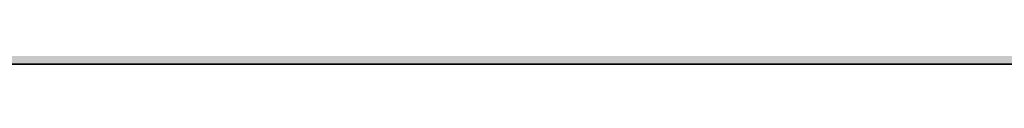
# Model space of a CAD drawing. Units: inches. Extents: x 2091 to 2899, y 967 to 2217.
# Tile 41 of 256: x 2390 to 2461, y 1091 to 1091. Entities that reach past the tile are written whole.
import ezdxf

# ---------------------------------------------------------------- set-up
doc = ezdxf.new("R2010")
doc.units = ezdxf.units.IN
doc.layers.add('A-WALL-PATT', color=141, linetype='Continuous', lineweight=13, true_color=0xadddf7)
doc.layers.add('C-PROP', color=7, linetype='Continuous', lineweight=35)

msp = doc.modelspace()

# ---------------------------------------------------------------- hatches: boundary and pattern name
at = {"layer": 'A-WALL-PATT'}
h = msp.add_hatch(color=256, dxfattribs=at)
h.dxf.hatch_style = 1
h.paths.add_polyline_path([(2212.144, 1941.419), (2387.644, 1941.419), (2387.644, 1824.419), (2392.144, 1824.419), (2392.144, 1941.419), (2609.644, 1941.419), (2609.644, 1825.919), (2614.144, 1825.919), (2614.144, 1941.419), (2794.144, 1941.419), (2794.144, 1928.762), (2803.144, 1928.762), (2803.144, 2050.919), (2203.144, 2050.919), (2203.144, 1900.758), (2212.144, 1900.758)])
h.paths.add_polyline_path([(2212.144, 1945.919), (2212.144, 2041.919), (2794.144, 2041.919), (2794.144, 1945.919), (2402.248, 1945.919), (2401.102, 1945.776), (2398.702, 1945.776)], flags=16)
h.paths.add_polyline_path([(2230.23, 1948.063), (2227.35, 1949.503), (2225.91, 1951.903), (2223.99, 1952.863), (2223.03, 1955.263), (2222.07, 1959.583), (2222.07, 1963.423), (2223.03, 1965.663), (2223.99, 1965.343), (2225.586, 1963.861), (2226.912, 1964.957), (2226.949, 1965.939), (2227.778, 1966.952), (2228.2, 1968.879), (2230.71, 1964.863), (2233.59, 1966.303), (2233.607, 1966.332), (2233.773, 1964.938), (2234.634, 1963.676), (2235.03, 1963.903), (2236.282, 1965.572), (2235.99, 1962.943), (2237.955, 1957.54), (2238.39, 1957.903), (2239.216, 1960.306), (2238.655, 1966.385), (2238.693, 1966.438), (2238.841, 1967.5), (2238.78, 1967.687), (2238.881, 1967.787), (2238.667, 1966.252), (2239.216, 1960.306), (2238.39, 1957.903), (2236.95, 1956.703), (2234.55, 1949.983)], flags=0)
h.paths.add_polyline_path([(2278.012, 1948.063), (2276.496, 1947.873), (2275.85, 1947.689), (2274.652, 1947.103)], flags=0)
h.paths.add_polyline_path([(2269.852, 1955.743), (2268.276, 1956.629), (2270.867, 1956.348), (2269.372, 1958.143), (2268.715, 1959.192), (2270.57, 1958.729), (2268.581, 1961.906), (2270.812, 1960.892), (2270.812, 1963.423), (2271.393, 1964.779), (2270.292, 1966.156), (2271.772, 1965.663), (2272.141, 1966.525), (2273.93, 1965.929), (2275.63, 1968.054), (2276.332, 1966.722), (2276.52, 1966.952), (2276.942, 1968.879), (2277.734, 1967.611), (2278.14, 1969.465), (2279.659, 1967.034), (2280.412, 1966.783), (2280.949, 1967.589), (2281.61, 1967.369), (2282.133, 1968.154), (2282.349, 1966.333), (2282.35, 1966.333), (2283.408, 1968.095), (2283.713, 1965.524), (2284.32, 1964.634), (2284.512, 1964.889), (2284.235, 1965.705), (2284.5, 1967.319), (2284.908, 1965.417), (2285.396, 1966.069), (2285.433, 1966.291), (2285.473, 1966.171), (2286.354, 1967.345), (2286.222, 1966.158), (2287.663, 1968.08), (2287.714, 1968.443), (2288.482, 1969.017), (2288.574, 1968.729), (2288.917, 1969.069), (2288.607, 1966.838), (2288.929, 1963.351), (2288.935, 1963.357), (2288.93, 1963.34), (2289.015, 1962.414), (2290.111, 1963.875), (2290.133, 1963.943), (2290.218, 1964.017), (2290.111, 1963.875), (2289.156, 1960.892), (2288.594, 1959.257), (2288.572, 1959.103), (2289.532, 1960.543), (2290.012, 1962.463), (2290.192, 1962.643), (2289.77, 1959.689), (2286.89, 1957.289), (2284.49, 1950.569), (2283.315, 1950.046), (2283.292, 1949.983), (2280.29, 1948.649), (2281.13, 1948.649), (2282.57, 1948.169), (2283.205, 1948.063), (2278.972, 1948.063), (2276.092, 1949.503), (2274.652, 1951.903), (2272.732, 1952.863)], flags=0)
h.paths.add_polyline_path([(2271.159, 1958.022), (2272.97, 1955.849), (2272.01, 1960.169), (2272.01, 1964.009), (2272.624, 1965.443), (2274.328, 1963.861), (2275.654, 1964.957), (2275.638, 1964.539), (2277.412, 1966.007), (2277.033, 1965.157), (2276.83, 1964.976), (2276.766, 1963.295), (2277.45, 1962.66), (2279.452, 1964.863), (2282.332, 1966.303), (2283.53, 1966.889), (2283.295, 1966.771), (2283.913, 1963.885), (2284.899, 1964.448), (2284.732, 1962.943), (2286.697, 1957.54), (2287.132, 1957.903), (2287.542, 1959.095), (2287.779, 1958.442), (2285.683, 1956.695), (2285.877, 1959.795), (2284.732, 1962.943), (2284.899, 1964.448), (2283.913, 1963.885), (2284.224, 1962.434), (2283.424, 1963.605), (2281.61, 1962.569), (2281.13, 1960.169), (2282.09, 1956.329), (2283.05, 1952.969), (2282.57, 1950.569), (2280.17, 1948.649), (2279.883, 1948.792), (2278.972, 1948.063), (2278.972, 1949.023), (2278.672, 1949.397), (2277.29, 1950.089), (2275.85, 1952.489), (2273.93, 1953.449), (2272.49, 1954.889), (2271.922, 1954.889), (2271.772, 1955.263)], flags=0)
h.paths.add_polyline_path([(2311.994, 1955.743), (2312.063, 1955.674), (2312.055, 1955.709)], flags=0)
h.paths.add_polyline_path([(2331.956, 1963.952), (2333.396, 1965.392), (2331.077, 1963.357), (2330.999, 1963.112)], flags=0)
h.paths.add_polyline_path([(2310.554, 1954.303), (2307.04, 1956.28), (2310.763, 1955.876), (2312.474, 1953.823), (2313.434, 1951.423), (2315.354, 1950.463), (2316.794, 1948.063), (2317.466, 1947.727), (2319.369, 1947.965), (2317.754, 1949.983), (2317.57, 1950.61), (2316.794, 1951.903), (2314.874, 1952.863), (2313.914, 1955.263), (2311.514, 1958.143), (2309.375, 1961.559), (2311.514, 1960.337), (2311.514, 1961.983), (2310.605, 1963.12), (2311.727, 1962.479), (2312.418, 1964.093), (2312.256, 1964.296), (2313.194, 1963.983), (2313.914, 1965.663), (2314.647, 1965.419), (2315.354, 1966.303), (2316.794, 1967.743), (2316.157, 1966.947), (2317.034, 1965.282), (2317.223, 1965.512), (2317.777, 1968.046), (2318.474, 1966.722), (2318.663, 1966.952), (2319.084, 1968.879), (2321.207, 1965.482), (2322.161, 1966.914), (2322.554, 1966.783), (2322.786, 1967.131), (2322.882, 1966.324), (2323.312, 1965.722), (2323.651, 1965.891), (2324.396, 1967.133), (2324.657, 1964.938), (2324.972, 1964.477), (2325.387, 1967.001), (2325.941, 1964.418), (2327.229, 1966.136), (2327.166, 1965.572), (2328.059, 1966.763), (2328.225, 1966.247), (2329.668, 1967.677), (2329.665, 1967.687), (2329.765, 1967.787), (2329.551, 1966.252), (2330.1, 1960.306), (2329.333, 1958.073), (2329.313, 1957.935), (2329.634, 1958.203), (2330.234, 1959.103), (2330.714, 1961.023), (2331.034, 1961.343), (2330.714, 1959.103), (2329.634, 1958.203), (2329.274, 1957.663), (2327.712, 1956.361), (2325.434, 1949.983), (2324.334, 1949.494), (2323.994, 1948.543), (2319.674, 1946.623), (2316.794, 1948.063), (2315.354, 1950.463), (2313.434, 1951.423)], flags=0)
h.paths.add_polyline_path([(2321.336, 1947.952), (2321.114, 1948.063), (2321.114, 1949.023), (2319.194, 1951.423), (2316.794, 1959.583), (2316.663, 1959.583), (2315.354, 1958.143), (2314.394, 1958.143), (2313.148, 1958.709), (2312.954, 1959.583), (2312.954, 1960.892), (2315.834, 1959.583), (2316.663, 1959.583), (2317.315, 1960.299), (2315.03, 1962.421), (2316.356, 1963.517), (2316.372, 1963.952), (2316.47, 1963.861), (2317.796, 1964.957), (2317.755, 1963.89), (2319.175, 1965.157), (2319.498, 1965.881), (2321.114, 1965.343), (2323.236, 1962.372), (2325.686, 1963.773), (2325.543, 1962.481), (2325.199, 1963.494), (2324.479, 1963.082), (2324.926, 1960.994), (2324.078, 1962.236), (2322.415, 1961.286), (2322.074, 1959.583), (2323.034, 1955.743), (2323.994, 1952.383), (2323.514, 1949.983), (2322.143, 1948.886), (2322.074, 1948.543)], flags=0)
h.paths.add_polyline_path([(2320.207, 1963.337), (2320.154, 1963.423), (2320.394, 1963.543)], flags=0)
h.paths.add_polyline_path([(2353.851, 1965.811), (2354.031, 1965.751), (2354.331, 1966.451), (2354.331, 1966.931)], flags=0)
h.paths.add_polyline_path([(2359.021, 1969.026), (2359.098, 1968.902), (2359.234, 1969.52), (2359.234, 1970)], flags=0)
h.paths.add_polyline_path([(2358.257, 1966.682), (2357.984, 1966.348), (2358.211, 1966.146), (2358.41, 1966.39)], flags=0)
h.paths.add_polyline_path([(2357.768, 1966.059), (2357.732, 1965.105), (2357.751, 1965.121), (2357.77, 1965.607), (2357.77, 1966.058)], flags=0)
h.paths.add_polyline_path([(2359.112, 1965.305), (2359.112, 1964.825), (2359.845, 1966.468), (2359.845, 1966.948)], flags=0)
h.paths.add_polyline_path([(2360.224, 1966.621), (2360.699, 1969.363), (2360.699, 1969.843), (2360.211, 1967.026), (2360.211, 1966.643)], flags=0)
h.paths.add_polyline_path([(2363.451, 1967.891), (2363.451, 1968.371), (2362.491, 1966.931), (2362.656, 1966.699)], flags=0)
h.paths.add_polyline_path([(2364.476, 1966.079), (2365.851, 1968.371), (2365.851, 1968.851), (2364.428, 1966.48)], flags=0)
h.paths.add_polyline_path([(2366.314, 1965.853), (2366.367, 1965.696), (2366.803, 1968.346), (2366.803, 1968.826)], flags=0)
h.paths.add_polyline_path([(2367.165, 1965.804), (2367.291, 1966.931), (2367.291, 1967.411), (2367.103, 1965.72)], flags=0)
h.paths.add_polyline_path([(2370.037, 1959.974), (2371.014, 1963.025), (2371.014, 1963.505), (2370.037, 1960.454)], flags=0)
h.paths.add_polyline_path([(2371.611, 1960.211), (2372.571, 1961.651), (2372.571, 1962.131), (2371.803, 1960.979)], flags=0)
h.paths.add_polyline_path([(2350.874, 1956.005), (2351.931, 1955.891), (2354.491, 1953.331), (2353.851, 1954.931), (2351.451, 1957.811), (2347.936, 1963.426), (2347.936, 1963.906), (2351.451, 1958.291), (2353.705, 1955.585), (2352.891, 1959.251), (2352.891, 1959.731), (2352.891, 1961.925), (2356.731, 1959.731), (2358.454, 1961.627), (2354.811, 1965.011), (2355.031, 1965.286), (2358.691, 1961.887), (2361.531, 1965.011), (2364.376, 1966.433), (2364.524, 1965.187), (2365.454, 1963.824), (2365.881, 1964.068), (2365.371, 1966.451), (2365.371, 1966.931), (2366.811, 1960.211), (2366.811, 1959.731), (2366.389, 1952.981), (2367.771, 1956.851), (2368.641, 1957.576), (2366.811, 1962.611), (2366.811, 1963.091), (2368.775, 1957.688), (2369.211, 1958.051), (2370.002, 1960.352), (2369.475, 1966.053), (2369.513, 1966.106), (2369.514, 1966.111), (2369.475, 1966.533), (2369.513, 1966.586), (2369.615, 1967.313), (2369.183, 1968.659), (2369.183, 1969.139), (2369.601, 1967.835), (2369.701, 1967.934), (2369.718, 1968.055), (2370.145, 1968.374), (2369.779, 1968.011), (2369.701, 1967.454), (2370.468, 1968.214), (2369.675, 1967.266), (2369.514, 1966.111), (2370.037, 1960.454), (2370.037, 1959.974), (2369.442, 1958.243), (2370.651, 1959.251), (2371.046, 1962.018), (2371.131, 1962.131), (2370.651, 1958.771), (2367.771, 1956.371), (2365.371, 1949.651), (2362.079, 1948.188), (2363.451, 1947.731), (2361.051, 1947.731), (2360.091, 1947.731), (2357.104, 1947.357), (2360.091, 1948.211), (2358.171, 1949.171), (2356.731, 1951.571), (2354.811, 1952.531), (2351.931, 1955.411)], flags=0)
h.paths.add_polyline_path([(2361.051, 1948.691), (2359.131, 1951.091), (2356.731, 1959.251), (2355.771, 1959.251), (2352.891, 1960.56), (2352.891, 1961.445), (2355.891, 1959.731), (2356.731, 1959.731), (2356.837, 1959.368), (2361.531, 1964.531), (2363.248, 1965.389), (2364.925, 1963.042), (2362.491, 1961.651), (2362.064, 1959.517), (2362.971, 1955.891), (2363.931, 1952.531), (2363.931, 1952.051), (2363.451, 1949.651), (2361.051, 1947.731)], flags=0)
h.paths.add_polyline_path([(2359.131, 1951.571), (2359.291, 1951.371), (2361.051, 1954.451), (2361.051, 1954.931)], flags=0)
h.paths.add_polyline_path([(2357.22, 1966.546), (2356.793, 1968.815), (2356.793, 1969.295), (2357.22, 1967.026)], flags=0)
h.paths.add_polyline_path([(2361.051, 1954.451), (2361.531, 1958.771), (2361.531, 1959.251), (2361.051, 1954.931)], flags=0)
h.paths.add_polyline_path([(2402.548, 1948.486), (2402.302, 1948.416), (2402.59, 1948.416)], flags=0)
h.paths.add_polyline_path([(2394.142, 1956.096), (2395.685, 1954.553), (2396.72, 1953.971), (2396.062, 1955.616), (2395.241, 1956.601), (2395.879, 1956.442), (2395.102, 1959.936), (2395.102, 1963.776), (2396.062, 1966.016), (2397.022, 1965.696), (2398.618, 1964.214), (2399.944, 1965.31), (2399.981, 1966.292), (2400.811, 1967.305), (2401.232, 1969.232), (2403.538, 1965.543), (2403.942, 1967.389), (2404.702, 1967.136), (2405.46, 1966.075), (2406.622, 1966.656), (2406.64, 1966.685), (2406.805, 1965.291), (2406.926, 1965.115), (2407.342, 1964.976), (2407.874, 1965.774), (2408.169, 1964.398), (2409.315, 1965.925), (2409.217, 1965.051), (2409.445, 1963.131), (2410.306, 1961.87), (2410.702, 1962.096), (2411.442, 1963.082), (2411.165, 1963.898), (2411.616, 1966.64), (2411.725, 1966.791), (2411.873, 1967.853), (2411.813, 1968.041), (2411.913, 1968.14), (2411.699, 1966.605), (2412.248, 1960.659), (2413.225, 1963.71), (2414.378, 1964.721), (2414.513, 1965.693), (2414.453, 1965.881), (2414.553, 1965.98), (2414.378, 1964.721), (2414.52, 1964.846), (2414.365, 1964.631), (2414.339, 1964.445), (2414.888, 1958.499), (2414.062, 1956.096), (2412.622, 1954.896), (2410.171, 1948.033), (2410.017, 1948.084), (2405.902, 1946.256), (2405.902, 1947.216), (2405.204, 1948.089), (2404.222, 1948.416), (2403.262, 1948.416), (2400.382, 1949.856), (2399.662, 1951.056), (2397.982, 1952.736), (2397.022, 1953.216), (2395.685, 1954.553), (2392.657, 1956.257)], flags=0)
h.paths.add_polyline_path([(2409.086, 1964.407), (2409.13, 1964.276), (2409.262, 1964.496)], flags=0)
h.paths.add_polyline_path([(2397.742, 1961.616), (2398.702, 1963.856), (2399.662, 1963.536), (2401.427, 1965.741), (2401.791, 1966.559), (2402.071, 1965.071), (2402.836, 1964.393), (2403.262, 1964.915), (2403.338, 1964.771), (2402.616, 1963.976), (2402.499, 1960.902), (2403.543, 1959.932), (2404.413, 1960.89), (2404.702, 1962.336), (2407.916, 1964.172), (2409.52, 1961.927), (2410.987, 1957.893), (2411.422, 1958.256), (2412.048, 1960.076), (2412.41, 1959.079), (2411.676, 1958.467), (2411.662, 1958.256), (2411.626, 1958.426), (2409.982, 1957.056), (2407.582, 1950.336), (2403.262, 1948.416), (2403.262, 1949.376), (2401.342, 1951.776), (2399.417, 1958.324), (2397.742, 1959.085), (2397.742, 1959.97), (2397.102, 1960.336), (2397.742, 1960.045)], flags=0)
h.paths.add_polyline_path([(2405.902, 1952.976), (2405.95, 1953.408), (2406.017, 1953.176)], flags=0)
h.paths.add_polyline_path([(2449.818, 1967.114), (2449.752, 1967.136), (2449.794, 1967.078)], flags=0)
h.paths.add_polyline_path([(2451.698, 1966.618), (2451.741, 1966.69), (2451.692, 1966.666)], flags=0)
h.paths.add_polyline_path([(2454.344, 1965.738), (2455.752, 1967.616), (2455.992, 1968.096), (2454.364, 1965.925)], flags=0)
h.paths.add_polyline_path([(2457.547, 1968.864), (2457.787, 1969.344), (2457.054, 1968.796), (2457.008, 1968.46)], flags=0)
h.paths.add_polyline_path([(2456.922, 1967.857), (2456.802, 1968.229), (2456.723, 1967.66)], flags=0)
h.paths.add_polyline_path([(2457.302, 1967.377), (2457.542, 1967.857), (2456.81, 1966.84), (2456.741, 1966.7), (2456.749, 1966.608)], flags=0)
h.paths.add_polyline_path([(2458.275, 1963.71), (2458.155, 1963.335), (2460.354, 1965.265), (2460.594, 1965.745)], flags=0)
h.paths.add_polyline_path([(2458.392, 1962.816), (2458.364, 1962.618), (2459.592, 1964.256), (2459.832, 1964.736)], flags=0)
h.paths.add_polyline_path([(2459.352, 1962.816), (2459.272, 1962.496), (2460.072, 1963.296), (2460.312, 1963.776)], flags=0)
h.paths.add_polyline_path([(2458.68, 1960.608), (2458.632, 1960.416), (2459.592, 1961.856), (2459.832, 1962.336)], flags=0)
h.paths.add_polyline_path([(2437.838, 1956.243), (2439.192, 1956.096), (2441.352, 1953.936), (2440.872, 1955.136), (2438.472, 1958.016), (2438.072, 1958.656), (2438.712, 1958.496), (2440.64, 1956.183), (2439.912, 1959.456), (2439.912, 1963.296), (2441.352, 1966.656), (2441.592, 1967.136), (2441.112, 1966.016), (2442.072, 1965.696), (2443.989, 1968.092), (2444.241, 1966.751), (2444.917, 1966.152), (2445.677, 1967.08), (2446.255, 1969.725), (2446.495, 1970.205), (2446.282, 1969.232), (2447.363, 1967.503), (2447.72, 1969.568), (2447.96, 1970.048), (2447.485, 1967.307), (2448.792, 1965.216), (2448.472, 1964.864), (2448.552, 1964.736), (2451.452, 1966.186), (2451.615, 1964.811), (2452.308, 1963.796), (2453.235, 1964.326), (2454.072, 1960.416), (2453.629, 1953.318), (2454.792, 1956.576), (2455.032, 1957.056), (2455.719, 1957.628), (2453.832, 1962.816), (2453.941, 1963.794), (2453.335, 1965.578), (2453.824, 1968.551), (2454.064, 1969.031), (2453.575, 1966.058), (2454.04, 1964.688), (2453.832, 1962.816), (2455.719, 1957.628), (2456.367, 1958.168), (2457.058, 1960.179), (2457.298, 1960.659), (2456.472, 1958.256), (2457.718, 1959.294), (2457.672, 1958.976), (2454.89, 1956.657), (2453.614, 1953.085), (2453.592, 1952.736), (2453.352, 1952.256), (2453.36, 1952.372), (2452.632, 1950.336), (2452.392, 1949.856), (2449.204, 1948.439), (2450.712, 1947.936), (2448.072, 1947.936), (2447.112, 1947.936), (2444.552, 1947.616), (2447.2, 1948.372), (2445.192, 1949.376), (2443.752, 1951.776), (2441.832, 1952.736), (2438.952, 1955.616)], flags=0)
h.paths.add_polyline_path([(2443.992, 1959.936), (2444.04, 1959.773), (2444.122, 1959.862)], flags=0)
h.paths.add_polyline_path([(2442.912, 1959.936), (2443.032, 1959.936), (2442.446, 1960.202)], flags=0)
h.paths.add_polyline_path([(2444.983, 1965.02), (2445.279, 1965.265), (2445.519, 1965.745), (2444.994, 1965.31)], flags=0)
h.paths.add_polyline_path([(2446.133, 1965.03), (2446.33, 1965.471), (2444.97, 1964.258), (2444.73, 1963.778)], flags=0)
h.paths.add_polyline_path([(2442.792, 1959.456), (2443.752, 1959.456), (2446.152, 1951.296), (2446.412, 1951.751), (2446.392, 1951.776), (2448.081, 1954.73), (2448.552, 1958.976), (2441.832, 1965.216), (2442.155, 1965.619), (2448.792, 1959.456), (2448.312, 1955.136), (2448.072, 1954.656), (2446.412, 1951.751), (2448.312, 1949.376), (2448.312, 1948.416), (2450.541, 1950.199), (2450.952, 1952.256), (2449.992, 1955.616), (2449.032, 1959.456), (2449.512, 1961.856), (2449.752, 1962.336), (2449.675, 1961.949), (2452.995, 1963.846), (2453.064, 1963.519), (2452.885, 1963.783), (2449.675, 1961.949), (2449.272, 1959.936), (2450.232, 1956.096), (2451.192, 1952.736), (2450.712, 1950.336), (2450.472, 1949.856), (2448.072, 1947.936), (2448.072, 1948.536), (2445.432, 1949.856), (2443.992, 1952.256), (2442.072, 1953.216), (2441.112, 1955.616), (2440.152, 1959.936), (2440.152, 1960.656)], flags=0)
h.paths.add_polyline_path([(2456.692, 1966.986), (2457.608, 1968.081), (2457.848, 1968.561), (2456.932, 1967.466)], flags=0)
h.paths.add_polyline_path([(2489.897, 1966.58), (2489.943, 1966.189), (2490.747, 1967.53), (2491.319, 1968.951)], flags=0)
h.paths.add_polyline_path([(2473.562, 1956.407), (2477.14, 1956.019), (2476.955, 1956.241), (2475.108, 1957.28), (2476.347, 1956.97), (2475.187, 1958.824), (2476.919, 1958.391), (2475.412, 1960.799), (2477.787, 1959.719), (2477.787, 1962.25), (2477.637, 1962.438), (2477.823, 1962.332), (2478.359, 1963.584), (2478.359, 1963.671), (2477.324, 1964.965), (2478.715, 1964.501), (2479.319, 1965.911), (2480.279, 1965.591), (2481.784, 1967.472), (2482.116, 1965.705), (2482.881, 1965.028), (2483.209, 1965.429), (2483.22, 1965.715), (2483.076, 1965.989), (2483.712, 1966.766), (2484.13, 1968.679), (2484.702, 1970.1), (2484.489, 1969.127), (2486.503, 1965.905), (2487.387, 1965.61), (2488.153, 1966.759), (2488.717, 1965.97), (2489.2, 1966.212), (2489.331, 1965.111), (2490.394, 1963.622), (2490.661, 1963.775), (2490.494, 1964.554), (2490.923, 1963.925), (2491.319, 1964.151), (2491.333, 1964.17), (2491.21, 1964.532), (2491.282, 1964.966), (2491.426, 1964.293), (2494.076, 1967.828), (2494.498, 1966.515), (2494.598, 1966.614), (2494.689, 1967.27), (2495.107, 1967.582), (2495.13, 1967.748), (2495.07, 1967.936), (2495.17, 1968.035), (2495.032, 1967.044), (2495.754, 1967.759), (2494.982, 1966.686), (2494.956, 1966.5), (2495.479, 1960.837), (2495.91, 1962.184), (2496.482, 1963.605), (2496.073, 1962.327), (2496.769, 1962.938), (2496.599, 1962.711), (2496.119, 1959.351), (2496.733, 1960.272), (2496.987, 1961.29), (2497.559, 1962.711), (2497.079, 1960.791), (2496.507, 1959.37), (2495.547, 1957.93), (2492.759, 1955.606), (2490.839, 1950.231), (2490.267, 1948.81), (2485.947, 1946.89), (2483.067, 1948.33), (2481.627, 1950.73), (2479.707, 1951.69), (2476.827, 1954.57)], flags=0)
h.paths.add_polyline_path([(2485.577, 1948.313), (2485.559, 1948.311), (2485.579, 1948.311)], flags=0)
h.paths.add_polyline_path([(2478.645, 1954.551), (2478.109, 1956.963), (2479.319, 1955.511), (2480.279, 1953.111), (2482.199, 1952.151), (2483.639, 1949.751), (2486.519, 1948.311), (2486.519, 1949.271), (2484.739, 1951.496), (2484.027, 1950.25), (2481.627, 1958.41), (2482.375, 1959.233), (2482.199, 1959.831), (2483.198, 1960.929), (2479.707, 1964.17), (2480.603, 1965.29), (2481.875, 1964.109), (2482.666, 1964.764), (2482.615, 1963.422), (2482.989, 1963.075), (2484.008, 1963.984), (2484.684, 1965.498), (2484.58, 1965.405), (2485.357, 1967.147), (2485.121, 1965.781), (2486.427, 1963.69), (2488.145, 1964.549), (2489.822, 1962.202), (2490.747, 1962.73), (2492, 1964.4), (2492.076, 1965.087), (2492.213, 1964.684), (2492.485, 1965.047), (2492.279, 1963.191), (2494.244, 1957.788), (2494.563, 1958.054), (2494.933, 1959.133), (2495.505, 1960.554), (2494.679, 1958.151), (2494.107, 1956.73), (2494.563, 1958.054), (2493.409, 1957.092), (2491.707, 1961.77), (2492, 1964.4), (2490.747, 1962.73), (2487.712, 1960.996), (2487.479, 1959.831), (2488.439, 1955.991), (2489.399, 1952.631), (2488.919, 1950.231), (2488.577, 1949.957), (2488.347, 1948.81), (2487.652, 1948.254), (2487.479, 1948.311), (2486.519, 1948.311), (2483.639, 1949.751), (2482.199, 1952.151), (2480.279, 1953.111), (2478.839, 1954.551)], flags=0)
h.paths.add_polyline_path([(2526.648, 1966.988), (2526.517, 1967.031), (2526.6, 1966.915)], flags=0)
h.paths.add_polyline_path([(2528.471, 1966.447), (2528.574, 1966.62), (2528.457, 1966.561)], flags=0)
h.paths.add_polyline_path([(2534.133, 1967.496), (2534.157, 1967.543), (2534.06, 1967.408)], flags=0)
h.paths.add_polyline_path([(2536.162, 1964.051), (2535.157, 1962.711), (2535.101, 1962.316), (2536.117, 1963.671), (2536.421, 1964.278)], flags=0)
h.paths.add_polyline_path([(2535.157, 1959.831), (2536.117, 1961.271), (2536.597, 1962.231), (2535.253, 1960.215)], flags=0)
h.paths.add_polyline_path([(2513.249, 1956.285), (2516.221, 1955.963), (2514.997, 1957.431), (2514.196, 1958.712), (2515.477, 1958.391), (2516.932, 1956.646), (2516.437, 1958.871), (2516.437, 1962.711), (2516.873, 1963.727), (2515.346, 1965.635), (2517.397, 1964.951), (2517.877, 1966.071), (2518.357, 1967.031), (2517.877, 1965.911), (2518.837, 1965.591), (2520.487, 1967.653), (2520.766, 1966.166), (2521.53, 1965.489), (2521.781, 1965.795), (2521.801, 1966.307), (2521.478, 1966.921), (2521.246, 1967.126), (2521.178, 1967.491), (2521.478, 1966.921), (2522.01, 1966.449), (2522.257, 1966.75), (2522.78, 1969.14), (2523.26, 1970.1), (2523.047, 1969.127), (2524.673, 1966.526), (2526.037, 1966.071), (2526.795, 1965.01), (2527.977, 1965.601), (2528.14, 1964.227), (2528.665, 1963.458), (2529.389, 1963.872), (2529.33, 1964.147), (2529.481, 1963.925), (2529.877, 1964.151), (2529.984, 1964.293), (2529.789, 1965.203), (2530.062, 1964.398), (2532.802, 1968.051), (2533.148, 1966.976), (2533.248, 1967.075), (2533.339, 1967.731), (2533.673, 1967.98), (2533.728, 1968.035), (2533.514, 1966.5), (2534.025, 1960.972), (2534.56, 1962.645), (2535.04, 1963.605), (2534.063, 1960.554), (2533.237, 1958.151), (2534.288, 1959.027), (2534.197, 1958.391), (2531.513, 1956.154), (2529.397, 1950.231), (2528.917, 1949.271), (2526.449, 1948.174), (2527.477, 1947.831), (2530.357, 1947.351), (2524.597, 1947.351), (2521.717, 1948.791), (2520.277, 1951.191), (2518.357, 1952.151), (2515.477, 1955.031)], flags=0)
h.paths.add_polyline_path([(2523.935, 1967.19), (2523.62, 1966.484), (2523.77, 1966.242)], flags=0)
h.paths.add_polyline_path([(2518.837, 1953.111), (2517.877, 1955.511), (2516.885, 1959.977), (2516.917, 1959.962), (2516.917, 1962.025), (2520.757, 1959.831), (2522.025, 1961.226), (2518.357, 1964.631), (2519.003, 1965.438), (2520.433, 1964.109), (2521.301, 1964.827), (2521.245, 1963.355), (2525.638, 1959.276), (2526.037, 1961.271), (2529.397, 1963.191), (2530.65, 1964.861), (2530.665, 1964.998), (2530.692, 1964.917), (2531.088, 1965.445), (2530.946, 1964.169), (2530.692, 1964.917), (2529.397, 1963.191), (2526.363, 1961.457), (2526.037, 1959.831), (2526.997, 1955.991), (2527.957, 1952.631), (2527.477, 1950.231), (2527.134, 1949.957), (2526.974, 1949.154), (2526.697, 1949.031), (2524.597, 1947.351), (2524.597, 1948.311), (2524.277, 1948.711), (2522.197, 1949.751), (2520.757, 1952.151)], flags=0)
h.paths.add_polyline_path([(2520.277, 1958.871), (2520.853, 1959.505), (2523.157, 1951.671), (2524.614, 1954.22), (2524.597, 1954.071), (2522.677, 1950.711)], flags=0)
h.paths.add_polyline_path([(2559.371, 1966.311), (2559.398, 1966.325), (2559.402, 1966.345)], flags=0)
h.paths.add_polyline_path([(2549.771, 1957.191), (2552.651, 1954.311), (2552.134, 1955.603), (2550.611, 1957.431), (2547.096, 1963.046), (2545.776, 1965.206), (2549.291, 1959.591), (2551.691, 1956.711), (2550.793, 1960.752), (2550.731, 1960.78), (2550.731, 1964.871), (2551.691, 1967.111), (2552.651, 1966.791), (2554.247, 1965.309), (2555.034, 1965.96), (2555.582, 1966.645), (2555.61, 1967.387), (2556.439, 1968.401), (2556.861, 1970.327), (2559.371, 1966.311), (2560.691, 1964.151), (2562.409, 1965.01), (2561.651, 1966.071), (2560.331, 1968.231), (2561.758, 1966.233), (2562.347, 1967.116), (2562.434, 1966.387), (2563.128, 1965.37), (2563.571, 1965.591), (2563.588, 1965.62), (2563.363, 1967.524), (2563.722, 1965.844), (2565.06, 1968.073), (2564.733, 1965.129), (2565.118, 1963.333), (2567.445, 1966.436), (2567.316, 1967.833), (2567.354, 1967.886), (2567.502, 1968.948), (2567.441, 1969.136), (2567.542, 1969.235), (2567.328, 1967.7), (2567.877, 1961.754), (2568.747, 1964.47), (2568.636, 1965.673), (2568.674, 1965.726), (2568.822, 1966.788), (2568.761, 1966.976), (2568.862, 1967.075), (2568.648, 1965.54), (2568.726, 1964.693), (2568.854, 1964.805), (2568.747, 1964.47), (2568.817, 1963.706), (2568.971, 1963.911), (2568.866, 1963.177), (2569.197, 1959.594), (2568.371, 1957.191), (2566.931, 1955.991), (2564.62, 1949.521), (2564.651, 1949.511), (2564.617, 1949.511), (2564.531, 1949.271), (2560.211, 1947.351), (2557.331, 1948.791), (2556.045, 1950.934), (2556.011, 1950.951), (2555.857, 1951.208), (2553.971, 1952.151), (2551.091, 1955.031), (2546.65, 1957.53)], flags=0)
h.paths.add_polyline_path([(2567.026, 1959.33), (2567.035, 1959.305), (2567.051, 1959.351)], flags=0)
h.paths.add_polyline_path([(2551.968, 1962.518), (2553.011, 1964.951), (2553.971, 1964.631), (2555.567, 1963.149), (2556.893, 1964.246), (2556.93, 1965.227), (2557.144, 1965.489), (2556.42, 1966.131), (2556.391, 1966.105), (2556.38, 1966.166), (2556.42, 1966.131), (2556.952, 1966.605), (2557.092, 1966.919), (2557.571, 1966.01), (2557.759, 1966.241), (2557.418, 1964.68), (2556.893, 1964.246), (2556.807, 1961.998), (2560.691, 1958.391), (2560.636, 1957.893), (2560.811, 1957.191), (2561.771, 1953.831), (2561.291, 1951.431), (2559.11, 1949.687), (2559.156, 1949.629), (2563.027, 1951.349), (2562.611, 1949.271), (2560.211, 1947.351), (2560.211, 1948.311), (2559.251, 1949.511), (2558.891, 1949.511), (2558.891, 1949.961), (2558.291, 1950.711), (2558.054, 1951.518), (2556.971, 1952.871), (2555.068, 1959.341), (2552.051, 1961.065), (2552.051, 1962.471)], flags=0)
h.paths.add_polyline_path([(2588.33, 1958.391), (2588.61, 1958.111), (2588.553, 1958.367)], flags=0)
h.paths.add_polyline_path([(2594.745, 1950.493), (2593.958, 1953.172), (2593.13, 1954.551), (2591.21, 1955.511), (2590.25, 1957.911), (2588.309, 1960.24), (2586.177, 1961.209), (2587.85, 1960.791), (2587.253, 1961.744), (2588.441, 1961.065), (2588.441, 1962.656), (2588.422, 1962.665), (2588.441, 1962.711), (2586.914, 1964.62), (2588.877, 1963.728), (2589.29, 1964.692), (2589.29, 1966.071), (2590.25, 1968.311), (2591.21, 1967.991), (2592.806, 1966.509), (2594.132, 1967.606), (2594.169, 1968.587), (2594.999, 1969.601), (2595.42, 1971.527), (2597.93, 1967.511), (2600.81, 1968.951), (2600.827, 1968.98), (2600.993, 1967.587), (2601.854, 1966.325), (2602.107, 1966.47), (2602.236, 1967.255), (2602.357, 1966.693), (2603.502, 1968.221), (2603.21, 1965.591), (2605.175, 1960.188), (2605.507, 1960.465), (2605.026, 1965.673), (2605.064, 1965.726), (2605.212, 1966.788), (2605.152, 1966.976), (2605.252, 1967.075), (2605.343, 1967.731), (2605.953, 1968.187), (2605.875, 1969.033), (2605.913, 1969.086), (2606.061, 1970.148), (2606, 1970.336), (2606.101, 1970.435), (2605.887, 1968.9), (2606.436, 1962.954), (2605.61, 1960.551), (2605.997, 1960.874), (2606.564, 1962.645), (2608.241, 1964.117), (2608.01, 1963.191), (2607.05, 1961.751), (2606.631, 1961.402), (2606.201, 1958.391), (2603.321, 1955.991), (2600.921, 1949.271), (2596.601, 1947.351), (2593.721, 1948.791), (2592.857, 1950.231), (2592.65, 1950.231)], flags=0)
h.paths.add_polyline_path([(2596.601, 1947.351), (2596.601, 1948.311), (2594.681, 1950.711), (2596.155, 1953.29), (2595.53, 1954.071), (2593.199, 1961.996), (2592.651, 1962.505), (2591.78, 1963.003), (2593.283, 1964.246), (2593.32, 1965.227), (2594.15, 1966.241), (2594.571, 1968.167), (2596.183, 1965.589), (2596.951, 1966.435), (2598.041, 1966.071), (2598.799, 1965.01), (2599.961, 1965.591), (2599.979, 1965.62), (2600.144, 1964.227), (2601.005, 1962.965), (2601.401, 1963.191), (2602.653, 1964.861), (2602.361, 1962.231), (2603.793, 1958.295), (2601.978, 1953.212), (2601.946, 1952.709), (2599.469, 1951.608), (2599.001, 1949.271)], flags=0)
h.paths.add_polyline_path([(2597.561, 1958.871), (2597.671, 1959.419), (2597.595, 1958.736)], flags=0)
h.paths.add_polyline_path([(2623.666, 1961.254), (2625.519, 1960.791), (2624.966, 1961.676), (2627.199, 1960.66), (2627.199, 1961.151), (2626.959, 1962.231), (2626.959, 1963.491), (2625.582, 1965.212), (2626.959, 1964.425), (2626.959, 1965.831), (2626.869, 1965.861), (2627.919, 1968.311), (2628.879, 1967.991), (2630.475, 1966.509), (2631.801, 1967.606), (2631.838, 1968.587), (2632.668, 1969.601), (2633.089, 1971.527), (2635.599, 1967.511), (2638.479, 1968.951), (2638.497, 1968.98), (2638.662, 1967.587), (2639.176, 1966.833), (2639.78, 1967.84), (2640.026, 1966.693), (2641.171, 1968.221), (2640.879, 1965.591), (2641.114, 1964.945), (2641.411, 1965.341), (2641.308, 1964.412), (2642.844, 1960.188), (2643.279, 1960.551), (2644.085, 1962.895), (2643.784, 1966.153), (2643.807, 1966.185), (2643.601, 1968.418), (2643.523, 1968.661), (2643.73, 1970.148), (2643.67, 1970.336), (2643.77, 1970.435), (2643.556, 1968.9), (2643.601, 1968.418), (2643.91, 1967.456), (2644.01, 1967.555), (2643.812, 1966.132), (2644.105, 1962.954), (2644.239, 1961.351), (2644.719, 1961.751), (2645.033, 1962.222), (2645.322, 1963.125), (2646.076, 1963.787), (2645.033, 1962.222), (2644.345, 1960.074), (2643.519, 1957.671), (2642.079, 1956.471), (2639.72, 1949.864), (2639.876, 1949.838), (2635.359, 1947.831), (2632.479, 1949.271), (2631.039, 1951.671), (2629.119, 1952.631), (2628.159, 1955.031), (2625.759, 1957.911)], flags=0)
h.paths.add_polyline_path([(2627.816, 1956.574), (2627.374, 1958.566), (2626.376, 1959.763), (2627.199, 1959.351), (2627.374, 1958.566), (2627.919, 1957.911), (2628.879, 1955.511), (2630.799, 1954.551), (2632.239, 1952.151), (2633.315, 1951.613), (2631.039, 1959.351), (2631.498, 1959.856), (2630.799, 1962.231), (2631.45, 1962.947), (2630.715, 1963.629), (2632.041, 1964.726), (2632.078, 1965.707), (2632.292, 1965.969), (2631.705, 1966.489), (2633.136, 1967.766), (2633.329, 1968.647), (2634.675, 1966.494), (2635.208, 1967.081), (2636.799, 1966.551), (2637.676, 1967.867), (2638.994, 1966.022), (2639.705, 1966.429), (2641.119, 1959.831), (2640.93, 1956.806), (2639.439, 1952.631), (2638.227, 1952.093), (2637.759, 1949.751), (2635.359, 1947.831), (2635.359, 1948.791), (2633.439, 1951.191), (2633.315, 1951.613), (2632.239, 1952.151), (2630.799, 1954.551), (2628.879, 1955.511)], flags=0)
h.paths.add_polyline_path([(2637.759, 1953.831), (2637.279, 1955.511), (2636.319, 1959.351), (2636.799, 1961.751), (2639.234, 1963.142), (2637.557, 1965.49), (2638.739, 1966.081), (2638.902, 1964.707), (2639.763, 1963.445), (2636.799, 1961.751), (2636.532, 1960.418), (2637.039, 1958.391), (2637.999, 1955.031)], flags=0)
h.paths.add_polyline_path([(2668.567, 1951.431), (2667.607, 1953.831), (2665.207, 1956.711), (2662.294, 1961.365), (2665.447, 1959.591), (2666.647, 1958.391), (2666.647, 1959.975), (2666.058, 1960.682), (2666.647, 1960.345), (2666.647, 1961.991), (2666.7, 1962.114), (2666.407, 1963.431), (2666.407, 1967.271), (2667.367, 1969.511), (2668.327, 1969.191), (2669.923, 1967.709), (2671.249, 1968.806), (2671.286, 1969.787), (2672.116, 1970.801), (2672.537, 1972.727), (2675.047, 1968.711), (2677.927, 1970.151), (2677.945, 1970.18), (2678.11, 1968.787), (2678.971, 1967.525), (2679.367, 1967.751), (2680.62, 1969.421), (2680.327, 1966.791), (2682.292, 1961.388), (2682.727, 1961.751), (2683.358, 1963.587), (2683.232, 1964.953), (2683.27, 1965.006), (2683.393, 1965.889), (2683.36, 1966.249), (2683.358, 1966.256), (2683.359, 1966.257), (2682.992, 1970.233), (2683.03, 1970.286), (2683.178, 1971.348), (2683.118, 1971.536), (2683.218, 1971.635), (2683.004, 1970.1), (2683.359, 1966.257), (2683.458, 1966.355), (2683.393, 1965.889), (2683.414, 1965.665), (2684.424, 1966.872), (2683.553, 1964.154), (2683.358, 1963.587), (2683.793, 1958.874), (2682.967, 1956.471), (2681.527, 1955.271), (2680.109, 1951.3), (2680.085, 1950.912), (2679.977, 1950.93), (2679.127, 1948.551), (2674.807, 1946.631), (2671.927, 1948.071), (2670.487, 1950.471)], flags=0)
h.paths.add_polyline_path([(2671.936, 1953.227), (2671.687, 1953.351), (2670.247, 1955.751), (2668.327, 1956.711), (2667.357, 1959.138), (2669.527, 1958.151), (2670.487, 1958.151), (2671.479, 1959.242), (2670.684, 1961.945), (2668.89, 1963.612), (2667.307, 1964.331), (2668.567, 1963.911), (2668.831, 1964.241), (2670.247, 1963.431), (2672.422, 1965.823), (2672.777, 1967.447), (2673.234, 1966.716), (2674.412, 1968.012), (2673.981, 1965.522), (2675.287, 1963.431), (2675.554, 1963.564), (2675.932, 1965.456), (2676.247, 1965.351), (2677.005, 1964.29), (2678.167, 1964.871), (2679.607, 1967.271), (2680.327, 1963.911), (2680.307, 1963.577), (2680.347, 1963.458), (2680.86, 1964.141), (2680.567, 1961.511), (2681.104, 1960.037), (2678.887, 1953.831), (2677.092, 1953.033), (2677.687, 1950.951), (2677.207, 1948.551), (2674.807, 1946.631), (2674.807, 1947.591), (2672.887, 1949.991)], flags=0)
h.paths.add_polyline_path([(2673.985, 1951.911), (2674.567, 1952.931), (2674.567, 1951.911), (2676.967, 1953.831), (2677.447, 1956.231), (2676.487, 1959.591), (2676.247, 1960.551), (2679.73, 1962.541), (2680.059, 1961.002), (2679.211, 1962.245), (2676.247, 1960.551), (2676.487, 1959.591), (2677.447, 1956.231), (2676.967, 1953.831), (2674.567, 1951.911)], flags=0)
h.paths.add_polyline_path([(2707.479, 1952.815), (2706.519, 1955.215), (2705.559, 1959.535), (2705.559, 1963.375), (2706.519, 1965.615), (2707.479, 1965.295), (2709.075, 1963.813), (2710.401, 1964.909), (2710.438, 1965.891), (2711.268, 1966.904), (2711.689, 1968.831), (2714.199, 1964.815), (2717.079, 1966.255), (2717.097, 1966.284), (2717.262, 1964.89), (2718.123, 1963.628), (2718.519, 1963.855), (2719.771, 1965.524), (2719.479, 1962.895), (2721.444, 1957.492), (2721.879, 1957.855), (2722.705, 1960.258), (2722.144, 1966.337), (2722.182, 1966.39), (2722.33, 1967.452), (2722.27, 1967.639), (2722.37, 1967.739), (2722.156, 1966.204), (2722.705, 1960.258), (2721.879, 1957.855), (2720.439, 1956.655), (2718.039, 1949.935), (2713.719, 1948.015), (2710.839, 1949.455), (2709.399, 1951.855)], flags=0)
h.paths.add_polyline_path([(2749.301, 1952.815), (2748.341, 1955.215), (2747.381, 1959.535), (2747.381, 1963.375), (2748.341, 1965.615), (2749.301, 1965.295), (2750.897, 1963.813), (2752.223, 1964.909), (2752.26, 1965.891), (2753.09, 1966.904), (2753.511, 1968.831), (2756.021, 1964.815), (2758.901, 1966.255), (2758.919, 1966.284), (2759.084, 1964.89), (2759.945, 1963.628), (2760.341, 1963.855), (2761.593, 1965.524), (2761.301, 1962.895), (2763.266, 1957.492), (2763.701, 1957.855), (2764.527, 1960.258), (2763.966, 1966.337), (2764.004, 1966.39), (2764.152, 1967.452), (2764.092, 1967.639), (2764.192, 1967.739), (2763.978, 1966.204), (2764.527, 1960.258), (2763.701, 1957.855), (2762.261, 1956.655), (2759.861, 1949.935), (2755.541, 1948.015), (2752.661, 1949.455), (2751.221, 1951.855)], flags=0)
h.paths.add_polyline_path([(2212.144, 1819.935), (2203.144, 1819.935), (2203.144, 1739.98), (2212.144, 1739.98), (2212.144, 1780.919), (2392.144, 1780.919), (2392.144, 1783.919), (2212.144, 1783.919)])
h.paths.add_polyline_path([(2803.144, 1847.939), (2794.144, 1847.939), (2794.144, 1785.419), (2609.644, 1785.419), (2493.876, 1785.419), (2493.876, 1780.919), (2609.644, 1780.919), (2794.144, 1780.919), (2794.144, 1696.919), (2609.376, 1696.919), (2609.376, 1742.919), (2604.876, 1742.919), (2604.876, 1644.419), (2609.376, 1644.419), (2609.376, 1692.419), (2794.144, 1692.419), (2794.144, 1668.165), (2803.144, 1668.165)])
h.paths.add_polyline_path([(2392.144, 1740.419), (2387.644, 1740.419), (2387.644, 1629.419), (2212.144, 1629.419), (2212.144, 1659.156), (2203.144, 1659.156), (2203.144, 1494.089), (2212.144, 1494.089), (2212.144, 1627.919), (2392.144, 1627.919)])
h.paths.add_polyline_path([(2457.876, 1780.919), (2453.376, 1780.919), (2453.376, 1644.419), (2568.876, 1644.419), (2568.876, 1648.919), (2457.876, 1648.919)])
h.paths.add_polyline_path([(2545.144, 1591.919), (2540.644, 1591.919), (2540.644, 1567.919), (2468.644, 1567.919), (2468.644, 1627.919), (2509.144, 1627.919), (2509.144, 1632.419), (2464.144, 1632.419), (2464.144, 1563.419), (2545.144, 1563.419)])
h.paths.add_polyline_path([(2268.644, 1555.919), (2212.144, 1555.919), (2212.144, 1551.419), (2268.644, 1551.419)], flags=17)
h.paths.add_polyline_path([(2212.144, 1413.266), (2203.144, 1413.266), (2203.144, 1233.07), (2212.144, 1233.07)])
h.paths.add_polyline_path([(2267.644, 1351.919), (2212.144, 1351.919), (2212.144, 1347.419), (2267.644, 1347.419)], flags=17)
h.paths.add_polyline_path([(2456.644, 1489.419), (2452.144, 1489.419), (2452.144, 1351.919), (2312.644, 1351.919), (2312.644, 1347.419), (2456.644, 1347.419)])
h.paths.add_polyline_path([(2472.37, 1455.419), (2467.87, 1455.419), (2467.87, 1347.419), (2472.37, 1347.419)])
h.paths.add_polyline_path([(2794.144, 1351.919), (2543.37, 1351.919), (2543.37, 1347.419), (2794.144, 1347.419)], flags=17)
h.paths.add_polyline_path([(2312.644, 1347.419), (2308.144, 1347.419), (2308.144, 1302.162), (2308.342, 1302.164), (2308.144, 1298.169), (2308.144, 1275.419), (2212.144, 1275.419), (2212.144, 1270.919), (2312.644, 1270.919)], flags=17)
h.paths.add_polyline_path([(2212.144, 1152.247), (2203.144, 1152.247), (2203.144, 1090.919), (2803.144, 1090.919), (2803.144, 1392.714), (2794.144, 1392.714), (2794.144, 1143.419), (2548.032, 1143.419), (2548.032, 1138.919), (2794.144, 1138.919), (2794.144, 1099.919), (2212.144, 1099.919)])
h.paths.add_polyline_path([(2471.532, 1266.329, 0.031658), (2467.032, 1269.946), (2467.032, 1143.419), (2471.532, 1143.419), (2471.532, 1148.819)], flags=17)
h.paths.add_polyline_path([(2803.144, 1587.341), (2794.144, 1587.341), (2794.144, 1473.537), (2803.144, 1473.537)])
h.paths.add_polyline_path([(2794.144, 1536.419), (2651.144, 1536.419), (2651.144, 1531.919), (2794.144, 1531.919)])
h.paths.add_polyline_path([(2614.144, 1620.419), (2609.644, 1620.419), (2609.644, 1536.419), (2614.144, 1536.419)])
h.paths.add_polyline_path([(2271.083, 1964.317), (2776.853, 1964.317), (2776.853, 2037.17), (2271.083, 2037.17)], flags=8)
h.paths.add_polyline_path([(2380.649, 1536.824), (2461.041, 1536.824), (2461.041, 1554.653), (2380.649, 1554.653)], flags=9)
h.paths.add_polyline_path([(2203.655, 1608.815), (2316.118, 1608.815), (2316.118, 1621.918), (2203.655, 1621.918)], flags=24)
h.paths.add_polyline_path([(2212.677, 1313.504), (2282.592, 1313.504), (2282.592, 1322.745), (2212.677, 1322.745)], flags=24)
h.paths.add_polyline_path([(2457.112, 1114.779), (2558.482, 1114.779), (2558.482, 1142.22), (2457.112, 1142.22)], flags=25)
h.paths.add_polyline_path([(2473.442, 1273.01), (2604.641, 1273.01), (2604.641, 1318.347), (2473.442, 1318.347)], flags=25)
h.paths.add_polyline_path([(2638.876, 1626.977), (2684.25, 1627.977), (2684.038, 1637.597), (2638.664, 1636.598)], flags=9)
h.paths.add_polyline_path([(2537.591, 1453.793), (2628.39, 1453.793), (2628.39, 1475.345), (2537.591, 1475.345)], flags=9)
h.paths.add_polyline_path([(2504.138, 1714.632), (2554.647, 1714.632), (2554.647, 1730.238), (2504.138, 1730.238)], flags=25)
h.paths.add_polyline_path([(2487.501, 1575.652), (2535.097, 1575.652), (2535.097, 1598.378), (2487.501, 1598.378)], flags=25)
h.paths.add_polyline_path([(2709.099, 1735.71), (2740.017, 1735.71), (2740.017, 1749.938), (2709.099, 1749.938)], flags=25)
h.paths.add_polyline_path([(2442.438, 1792.172), (2564.729, 1792.172), (2564.729, 1842), (2442.438, 1842)], flags=9)
h.paths.add_polyline_path([(2655.816, 1809.644), (2789.52, 1806.694), (2790.085, 1832.292), (2656.381, 1835.242)], flags=25)
h.paths.add_polyline_path([(2234.843, 1797.72), (2368.593, 1794.769), (2369.161, 1820.504), (2235.411, 1823.455)], flags=9)
h.paths.add_polyline_path([(2245.138, 1644.006), (2398.428, 1640.624), (2398.995, 1666.325), (2245.706, 1669.707)], flags=9)
h.paths.add_polyline_path([(2306.143, 1431.169), (2413.768, 1428.794), (2414.333, 1454.392), (2306.708, 1456.766)], flags=9)
h.paths.add_polyline_path([(2306.835, 1458.233), (2393.38, 1456.323), (2393.933, 1481.354), (2307.387, 1483.264)], flags=9)

# ---------------------------------------------------------------- linework, layer by layer
at = {"layer": 'C-PROP'}
msp.add_lwpolyline([(2203.144, 2050.919), (2803.144, 2050.919), (2803.144, 1090.919), (2203.144, 1090.919)], close=True, dxfattribs=at)

doc.saveas('drawing.dxf')
